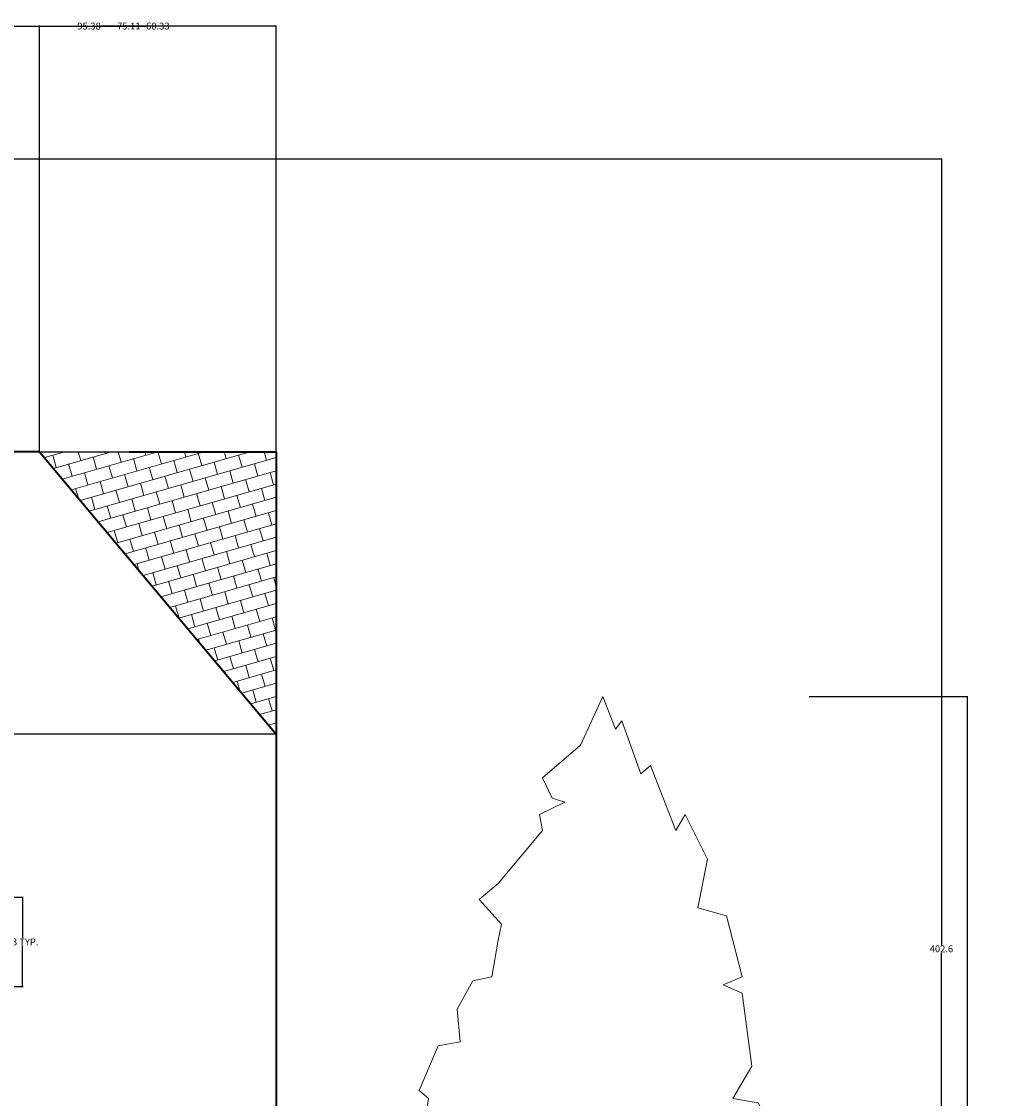
# Model space of a CAD drawing. Units: inches. Extents: x -17 to 741, y 7 to 490.
# Tile 8 of 8: x 489 to 741, y 215 to 490. Entities that reach past the tile are written whole.
import ezdxf

# ---------------------------------------------------------------- set-up
doc = ezdxf.new("R2010")
doc.units = ezdxf.units.IN
doc.header["$MEASUREMENT"] = 0
for name, color, linetype, lineweight in [('A-ANNO-DIMS', 2, 'Continuous', 18), ('A-ROOF-PATT', 8, 'Continuous', 13), ('A-WALL', 7, 'Continuous', 35), ('A-WALL-TRIM', 7, 'Continuous', 25), ('L-PLNT', 3, 'Continuous', 18)]:
    doc.layers.add(name, color=color, linetype=linetype, lineweight=lineweight)
doc.styles.get("Standard").update_dxf_attribs({"font": 'arial.ttf'})
doc.dimstyles.get("Standard").update_dxf_attribs({"dimtxt": 1.75, "dimasz": 0.18, "dimexe": 0.18, "dimexo": 0.0625, "dimgap": 0.09, "dimtad": 0, "dimtih": 1, "dimtoh": 1, "dimdec": 4, "dimzin": 0, "dimdsep": 46, "dimlunit": 4, "dimtxsty": 'Standard', "dimcen": 0.09, "dimadec": 0, "dimazin": 0, "dimtfac": 1, "dimtdec": 4, "dimtofl": 0, "dimtmove": 0, "dimatfit": 3, "dimfxl": 1, "dimtolj": 1, "dimtzin": 0, "dimarcsym": 0})

# ---------------------------------------------------------------- blocks, each defined once
blk = doc.blocks.new('Tree - type 2 deciduous elevation')
blk.add_lwpolyline([(-2.754, 191.699), (-6.78, 182.851), (-13.682, 176.953), (-11.956, 173.266), (-9.656, 172.529), (-14.257, 170.317), (-13.682, 167.368), (-21.733, 157.783), (-25.184, 154.834), (-21.158, 150.41), (-21.733, 147.461), (-22.884, 140.825), (-26.334, 140.087), (-29.21, 134.926), (-28.635, 129.028), (-32.661, 128.291), (-36.111, 120.18), (-34.386, 118.706), (-35.536, 111.333), (-38.987, 106.171), (-34.386, 107.646), (-40.712, 98.798), (-37.261, 95.849), (-40.712, 90.688), (-41.287, 80.366), (-38.412, 78.154), (-36.686, 70.781), (-39.562, 71.518), (-37.261, 64.145), (-38.412, 57.509), (-36.111, 58.247), (-33.236, 52.348), (-35.536, 53.086), (-34.961, 46.45), (-30.36, 44.975), (-31.51, 36.128), (-26.334, 36.865), (-23.459, 39.814), (-18.283, 36.128), (-20.008, 33.178), (-14.832, 31.704), (-11.956, 33.178), (-12.531, 27.28), (-6.205, 22.856), (-3.905, 24.331), (0.121, 22.856), (8.173, 26.543), (11.624, 25.068), (12.199, 27.28), (21.4, 34.653), (19.675, 39.077), (23.701, 44.975), (30.027, 47.924), (30.602, 53.823), (25.426, 56.772), (32.903, 61.196), (34.053, 67.094), (30.602, 75.205), (34.628, 89.951), (26.576, 103.222), (23.701, 103.222), (28.302, 107.646), (23.701, 110.595), (26.576, 115.756), (25.426, 117.968), (20.825, 118.706), (24.276, 124.604), (22.551, 137.876), (19.1, 139.35), (22.551, 140.825), (19.675, 151.884), (14.499, 153.359), (16.224, 162.207), (12.199, 170.317), (10.473, 167.368), (5.872, 179.165), (4.147, 177.69), (0.696, 187.275), (-0.454, 185.8)], close=True)
for points in [[(-6.813, 23.669), (-6.813, 11.669), (-8.627, 0)], [(0.387, 23.669), (-0.576, 13.271), (-0.576, 3.686), (0, 0)]]:
    blk.add_lwpolyline(points)
blk = doc.blocks.new('*D32')
at = {"layer": 'A-ANNO-DIMS', "color": 0, "lineweight": -2, "transparency": 16777216}
for p, q in [((484.78, 266.43), (489, 266.43)), ((488.82, 266.25), (488.82, 256.04)), ((488.82, 243.86), (488.82, 254.07)), ((484.78, 243.68), (489, 243.68))]:
    blk.add_line(p, q, dxfattribs=at)
at = {"layer": 'A-ANNO-DIMS', "color": 0, "transparency": 16777216}
for points in [[(488.79, 266.25), (488.85, 266.25), (488.82, 266.43)], [(488.79, 243.86), (488.85, 243.86), (488.82, 243.68)]]:
    blk.add_solid(points, dxfattribs=at)
at = {"layer": 'Defpoints', "color": 0, "transparency": 16777216}
for p in [(484.72, 266.43), (488.82, 266.43), (484.72, 243.68)]:
    blk.add_point(p, dxfattribs=at)
at = {"layer": 'A-ANNO-DIMS', "color": 0, "transparency": 16777216, "insert": (488.82, 255.05), "char_height": 1.75, "attachment_point": 5}
blk.add_mtext('\\A1;23 TYP.', dxfattribs=at)
blk = doc.blocks.new('*D35')
at = {"layer": 'A-ANNO-DIMS', "color": 0, "lineweight": -2, "transparency": 16777216}
for p, q in [((689.15, 317.56), (729.61, 317.56)), ((729.43, 317.38), (729.43, 184.06)), ((729.43, 48.74), (729.43, 182.06)), ((689.15, 48.56), (729.61, 48.56))]:
    blk.add_line(p, q, dxfattribs=at)
at = {"layer": 'A-ANNO-DIMS', "color": 0, "transparency": 16777216}
for points in [[(729.4, 317.38), (729.46, 317.38), (729.43, 317.56)], [(729.4, 48.74), (729.46, 48.74), (729.43, 48.56)]]:
    blk.add_solid(points, dxfattribs=at)
at = {"layer": 'Defpoints', "color": 0, "transparency": 16777216}
for p in [(689.08, 317.56), (729.43, 317.56), (689.08, 48.56)]:
    blk.add_point(p, dxfattribs=at)
at = {"layer": 'A-ANNO-DIMS', "color": 0, "transparency": 16777216, "insert": (729.43, 183.06), "char_height": 1.75, "attachment_point": 5}
blk.add_mtext('\\A1;DECIDUOUS TREE 269', dxfattribs=at)
blk = doc.blocks.new('*D37')
at = {"layer": 'A-ANNO-DIMS', "color": 0, "lineweight": -2, "transparency": 16777216}
for p, q in [((20.52, 396.95), (20.52, 14.58)), ((553.43, 51.95), (553.43, 14.58)), ((20.7, 14.76), (283.93, 14.76)), ((553.25, 14.76), (290.02, 14.76))]:
    blk.add_line(p, q, dxfattribs=at)
at = {"layer": 'A-ANNO-DIMS', "color": 0, "transparency": 16777216}
for points in [[(20.7, 14.79), (20.7, 14.73), (20.52, 14.76)], [(553.25, 14.79), (553.25, 14.73), (553.43, 14.76)]]:
    blk.add_solid(points, dxfattribs=at)
at = {"layer": 'Defpoints', "color": 0, "transparency": 16777216}
for p in [(20.52, 397.01), (553.43, 52.01), (553.43, 14.76)]:
    blk.add_point(p, dxfattribs=at)
at = {"layer": 'A-ANNO-DIMS', "color": 0, "transparency": 16777216, "insert": (286.97, 14.76), "char_height": 1.75, "attachment_point": 5}
blk.add_mtext('\\A1;532.9', dxfattribs=at)
blk = doc.blocks.new('*D38')
at = {"layer": 'A-ANNO-DIMS', "color": 0, "lineweight": -2, "transparency": 16777216}
for p, q in [((341.83, 454.57), (723.06, 454.57)), ((722.88, 454.39), (722.88, 254.27)), ((722.88, 52.19), (722.88, 252.31)), ((553.49, 52.01), (723.06, 52.01))]:
    blk.add_line(p, q, dxfattribs=at)
at = {"layer": 'A-ANNO-DIMS', "color": 0, "transparency": 16777216}
for points in [[(722.85, 454.39), (722.91, 454.39), (722.88, 454.57)], [(722.85, 52.19), (722.91, 52.19), (722.88, 52.01)]]:
    blk.add_solid(points, dxfattribs=at)
at = {"layer": 'Defpoints', "color": 0, "transparency": 16777216}
for p in [(341.77, 454.57), (722.88, 454.57), (553.43, 52.01)]:
    blk.add_point(p, dxfattribs=at)
at = {"layer": 'A-ANNO-DIMS', "color": 0, "transparency": 16777216, "insert": (722.88, 253.29), "char_height": 1.75, "attachment_point": 5}
blk.add_mtext('\\A1;402.6', dxfattribs=at)
blk = doc.blocks.new('*D46')
at = {"layer": 'A-ANNO-DIMS', "color": 0, "lineweight": -2, "transparency": 16777216}
for p, q in [((493.1, 380.01), (493.1, 488.55)), ((493.28, 488.37), (520.21, 488.37)), ((553.25, 488.37), (526.31, 488.37)), ((553.43, 380.01), (553.43, 488.55))]:
    blk.add_line(p, q, dxfattribs=at)
at = {"layer": 'A-ANNO-DIMS', "color": 0, "transparency": 16777216}
for points in [[(493.28, 488.4), (493.28, 488.34), (493.1, 488.37)], [(553.25, 488.4), (553.25, 488.34), (553.43, 488.37)]]:
    blk.add_solid(points, dxfattribs=at)
at = {"layer": 'Defpoints', "color": 0, "transparency": 16777216}
for p in [(493.1, 488.37), (493.1, 379.95), (553.43, 379.95)]:
    blk.add_point(p, dxfattribs=at)
at = {"layer": 'A-ANNO-DIMS', "color": 0, "transparency": 16777216, "insert": (523.26, 488.37), "char_height": 1.75, "attachment_point": 5}
blk.add_mtext('\\A1;60.33', dxfattribs=at)
blk = doc.blocks.new('*D47')
at = {"layer": 'A-ANNO-DIMS', "color": 0, "lineweight": -2, "transparency": 16777216}
for p, q in [((493.03, 379.95), (-13.46, 379.95)), ((-13.28, 379.77), (-13.28, 344.94)), ((-13.28, 308.15), (-13.28, 342.97)), ((553.37, 307.97), (-13.46, 307.97))]:
    blk.add_line(p, q, dxfattribs=at)
at = {"layer": 'A-ANNO-DIMS', "color": 0, "transparency": 16777216}
for points in [[(-13.31, 379.77), (-13.25, 379.77), (-13.28, 379.95)], [(-13.31, 308.15), (-13.25, 308.15), (-13.28, 307.97)]]:
    blk.add_solid(points, dxfattribs=at)
at = {"layer": 'Defpoints', "color": 0, "transparency": 16777216}
for p in [(493.1, 379.95), (-13.28, 307.97), (553.43, 307.97)]:
    blk.add_point(p, dxfattribs=at)
at = {"layer": 'A-ANNO-DIMS', "color": 0, "transparency": 16777216, "insert": (-13.28, 343.96), "char_height": 1.75, "attachment_point": 5}
blk.add_mtext('\\A1;71.98', dxfattribs=at)
blk = doc.blocks.new('*D54')
at = {"layer": 'A-ANNO-DIMS', "color": 0, "lineweight": -2, "transparency": 16777216}
for p, q in [((458.05, 167.89), (458.05, 488.55)), ((458.23, 488.37), (502.69, 488.37)), ((553.25, 488.37), (508.78, 488.37)), ((553.43, 52.07), (553.43, 488.55))]:
    blk.add_line(p, q, dxfattribs=at)
at = {"layer": 'A-ANNO-DIMS', "color": 0, "transparency": 16777216}
for points in [[(458.23, 488.4), (458.23, 488.34), (458.05, 488.37)], [(553.25, 488.4), (553.25, 488.34), (553.43, 488.37)]]:
    blk.add_solid(points, dxfattribs=at)
at = {"layer": 'Defpoints', "color": 0, "transparency": 16777216}
for p in [(553.43, 488.37), (458.05, 167.83), (553.43, 52.01)]:
    blk.add_point(p, dxfattribs=at)
at = {"layer": 'A-ANNO-DIMS', "color": 0, "transparency": 16777216, "insert": (505.74, 488.37), "char_height": 1.75, "attachment_point": 5}
blk.add_mtext('\\A1;95.38', dxfattribs=at)
blk = doc.blocks.new('*D65')
at = {"layer": 'A-ANNO-DIMS', "color": 0, "lineweight": -2, "transparency": 16777216}
for p, q in [((478.32, 220.07), (478.32, 488.55)), ((478.5, 488.37), (513.01, 488.37)), ((553.25, 488.37), (518.74, 488.37)), ((553.43, 308.03), (553.43, 488.55))]:
    blk.add_line(p, q, dxfattribs=at)
at = {"layer": 'A-ANNO-DIMS', "color": 0, "transparency": 16777216}
for points in [[(478.5, 488.4), (478.5, 488.34), (478.32, 488.37)], [(553.25, 488.4), (553.25, 488.34), (553.43, 488.37)]]:
    blk.add_solid(points, dxfattribs=at)
at = {"layer": 'Defpoints', "color": 0, "transparency": 16777216}
for p in [(553.43, 488.37), (553.43, 307.97), (478.32, 220.01)]:
    blk.add_point(p, dxfattribs=at)
at = {"layer": 'A-ANNO-DIMS', "color": 0, "transparency": 16777216, "insert": (515.87, 488.37), "char_height": 1.75, "attachment_point": 5}
blk.add_mtext('\\A1;75.11', dxfattribs=at)

msp = doc.modelspace()

# ---------------------------------------------------------------- hatches: boundary and pattern name
at = {"layer": 'A-ROOF-PATT'}
h = msp.add_hatch(dxfattribs=at)
h.set_pattern_fill('BRICK', color=256, scale=13, angle=16)
h.paths.add_polyline_path([(341.7687, 454.5717), (262.0821, 409.8217), (421.4553, 409.8217)])
h.paths.add_polyline_path([(553.4286, 379.9466), (515.96, 379.9466), (493.0961, 379.9466), (553.4286, 307.9703)])

# ---------------------------------------------------------------- linework, layer by layer
at = {"layer": 'A-WALL'}
for p, q in [((493.0961, 379.9466), (553.4286, 307.9703)), ((515.96, 379.9466), (553.4286, 379.9466)), ((553.4286, 379.9466), (553.4286, 52.0082))]:
    msp.add_line(p, q, dxfattribs=at)
at = {"layer": 'A-WALL-TRIM'}
msp.add_lwpolyline([(53.4591, 295.9), (53.4591, 295.9), (72.6093, 295.9), (97.1425, 365.3552), (97.1425, 379.9466), (515.96, 379.9466)], dxfattribs=at)

# ---------------------------------------------------------------- block references
at = {"layer": 'L-PLNT', "xscale": 1.403243224327764, "yscale": 1.403243224327764, "zscale": 1.403243224327764}
msp.add_blockref('Tree - type 2 deciduous elevation', (640.4911, 48.5597), dxfattribs=at)

# ---------------------------------------------------------------- dimensions: what is measured, and where the dimension line sits
at = {"layer": 'A-ANNO-DIMS'}
for base, p1, p2, override, picture, middle in [((553.4286, 488.3717), (458.0494, 167.8255), (553.4286, 52.0082), {"dimdec": 2, "dimlfac": 1, "dimrnd": 0, "dimzin": 0, "dimdsep": 46, "dimlunit": 2}, '*D54', (505.739, 488.3717)), ((553.4286, 488.3717), (478.3168, 220.0082), (553.4286, 307.9703), {"dimdec": 2, "dimlfac": 1, "dimrnd": 0, "dimzin": 0, "dimdsep": 46, "dimlunit": 2}, '*D65', (515.8727, 488.3717)), ((493.0961, 488.3717), (553.4286, 379.9466), (493.0961, 379.9466), {"dimdec": 2, "dimlfac": 1, "dimrnd": 0, "dimzin": 0, "dimdsep": 46, "dimlunit": 2}, '*D46', (523.2623, 488.3717)), ((553.4286, 14.7597), (20.5169, 397.0087), (553.4286, 52.0082), {"dimdec": 1, "dimlfac": 1, "dimrnd": 0, "dimzin": 0, "dimdsep": 46, "dimlunit": 2}, '*D37', (286.9727, 14.7597))]:
    dim = msp.add_linear_dim(base=base, p1=p1, p2=p2, dimstyle='Standard', override=override, dxfattribs=at)
    dim.commit()
    dim.dimension.update_dxf_attribs({"geometry": picture, "text_midpoint": middle})
for base, p1, p2, override, picture, middle in [((722.8826, 454.5717), (553.4286, 52.0082), (341.7687, 454.5717), {"dimdec": 1, "dimlfac": 1, "dimrnd": 0, "dimzin": 0, "dimdsep": 46, "dimlunit": 2}, '*D38', (722.8826, 253.2899)), ((-13.2831, 307.9703), (493.0961, 379.9466), (553.4286, 307.9703), {"dimdec": 2, "dimlfac": 1, "dimrnd": 0, "dimzin": 0, "dimdsep": 46, "dimlunit": 2}, '*D47', (-13.2831, 343.9584))]:
    dim = msp.add_linear_dim(base=base, p1=p1, p2=p2, angle=90, dimstyle='Standard', override=override, dxfattribs=at)
    dim.commit()
    dim.dimension.update_dxf_attribs({"geometry": picture, "text_midpoint": middle})
for base, p1, p2, text, picture, middle in [((729.4326, 317.56), (689.0826, 48.5597), (689.0826, 317.56), 'DECIDUOUS TREE <>', '*D35', (729.4326, 183.0598)), ((488.8154, 266.4257), (484.7197, 243.6767), (484.7197, 266.4257), '<> TYP.', '*D32', (488.8154, 255.0512))]:
    dim = msp.add_linear_dim(base=base, p1=p1, p2=p2, angle=90, text=text, dimstyle='Standard', override={"dimdec": 0, "dimlfac": 1, "dimrnd": 0, "dimzin": 0, "dimdsep": 46, "dimlunit": 2}, dxfattribs=at)
    dim.commit()
    dim.dimension.update_dxf_attribs({"geometry": picture, "text_midpoint": middle})

doc.saveas('drawing.dxf')
